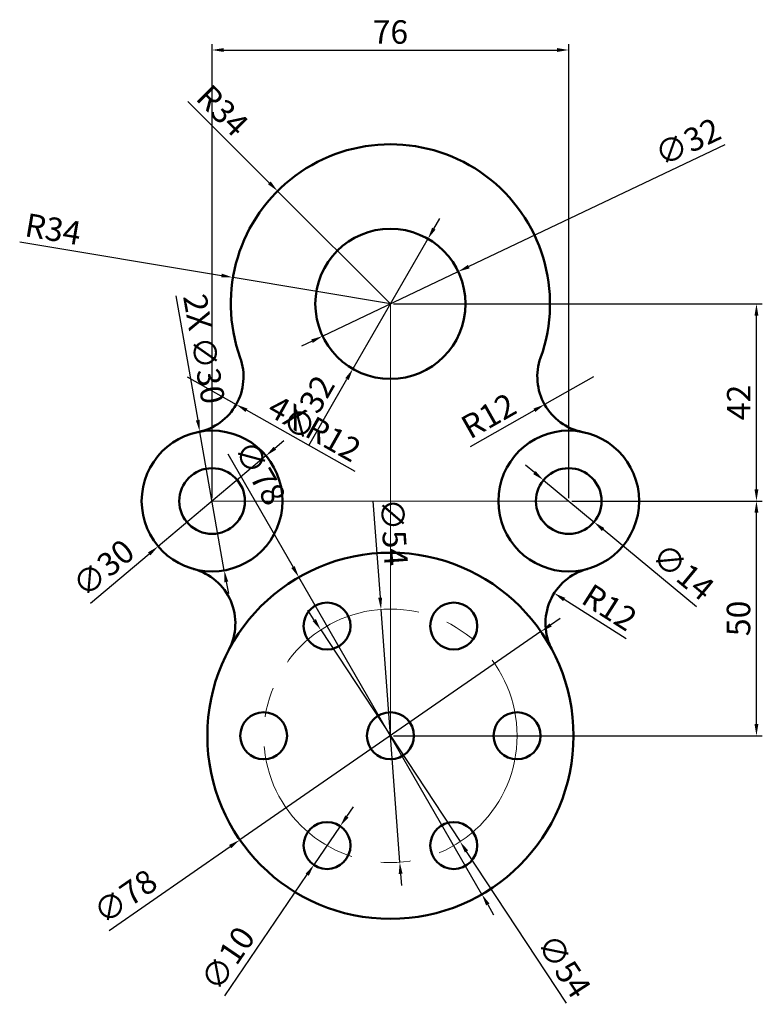
# Model space of a CAD drawing. Units: millimetres. Extents: x 2281 to 2439, y 1720 to 1930.
import ezdxf

# ---------------------------------------------------------------- set-up
doc = ezdxf.new("R2010")
doc.units = ezdxf.units.MM
doc.linetypes.add('CENTER', pattern=[50.8, 31.75, -6.35, 6.35, -6.35])
for name, color, linetype, lineweight in [('M-CNTR', 4, 'CENTER', 18), ('M-CONS', 8, 'Continuous', 13), ('M-DIMS', 2, 'Continuous', 25), ('M-OUTL', 7, 'Continuous', 50)]:
    doc.layers.add(name, color=color, linetype=linetype, lineweight=lineweight)
doc.styles.get("Standard").update_dxf_attribs({"font": 'arial.ttf'})
doc.dimstyles.new('ISO-25', dxfattribs={"dimtxt": 5, "dimasz": 2.5, "dimexe": 1.25, "dimexo": 0.625, "dimtad": 1, "dimtxsty": 'Standard', "dimcen": 2.5, "dimadec": 0, "dimazin": 0, "dimtfac": 1, "dimtmove": 0, "dimatfit": 3, "dimfxl": 1, "dimarcsym": 0})

# ---------------------------------------------------------------- blocks, each defined once
blk = doc.blocks.new('*U1')
blk.add_circle((0, 0), 5)
blk = doc.blocks.new('*U2')
at = {"layer": 'M-OUTL', "color": 0, "linetype": 'ByBlock', "lineweight": -2, "transparency": 16777216}
for p, rotation in [((2346.54, 1801.05), 119.9999999999999), ((2373.54, 1801.05), 59.99999999999997), ((2333.04, 1777.67), 180), ((2346.54, 1754.29), 239.9999999999999), ((2373.54, 1754.29), 299.9999999999999)]:
    blk.add_blockref('*U1', p, dxfattribs=dict(at, rotation=rotation))
blk.add_blockref('*U1', (2387.04, 1777.67), dxfattribs=at)
blk = doc.blocks.new('*D3')
at = {"layer": 'Defpoints', "color": 0, "transparency": 16777216}
for p in [(2398.04, 1923.75), (2322.04, 1827.67), (2398.04, 1827.67)]:
    blk.add_point(p, dxfattribs=at)
at = {"layer": 'M-DIMS', "color": 0, "lineweight": -2, "transparency": 16777216}
for p, q in [((2322.04, 1828.29), (2322.04, 1925)), ((2324.54, 1923.75), (2395.54, 1923.75)), ((2398.04, 1828.29), (2398.04, 1925))]:
    blk.add_line(p, q, dxfattribs=at)
at = {"layer": 'M-DIMS', "color": 0, "transparency": 16777216}
for points in [[(2324.54, 1924.16), (2324.54, 1923.33), (2322.04, 1923.75)], [(2395.54, 1924.16), (2395.54, 1923.33), (2398.04, 1923.75)]]:
    blk.add_solid(points, dxfattribs=at)
at = {"layer": 'M-DIMS', "color": 0, "transparency": 16777216, "insert": (2360.04, 1926.93), "char_height": 5, "attachment_point": 5}
blk.add_mtext('76', dxfattribs=at)
blk = doc.blocks.new('*D4')
at = {"layer": 'Defpoints', "color": 0, "transparency": 16777216}
for p in [(2398.04, 1827.67), (2438.04, 1827.67), (2360.04, 1777.67)]:
    blk.add_point(p, dxfattribs=at)
at = {"layer": 'M-DIMS', "color": 0, "lineweight": -2, "transparency": 16777216}
for p, q in [((2398.67, 1827.67), (2439.29, 1827.67)), ((2438.04, 1780.17), (2438.04, 1825.17)), ((2360.67, 1777.67), (2439.29, 1777.67))]:
    blk.add_line(p, q, dxfattribs=at)
at = {"layer": 'M-DIMS', "color": 0, "transparency": 16777216}
for points in [[(2437.62, 1825.17), (2438.45, 1825.17), (2438.04, 1827.67)], [(2437.62, 1780.17), (2438.45, 1780.17), (2438.04, 1777.67)]]:
    blk.add_solid(points, dxfattribs=at)
at = {"layer": 'M-DIMS', "color": 0, "transparency": 16777216, "insert": (2434.86, 1802.67), "char_height": 5, "attachment_point": 5, "rotation": 90}
blk.add_mtext('50', dxfattribs=at)
blk = doc.blocks.new('*D5')
at = {"layer": 'Defpoints', "color": 0, "transparency": 16777216}
for p in [(2360.04, 1869.67), (2438.04, 1869.67), (2398.04, 1827.67)]:
    blk.add_point(p, dxfattribs=at)
at = {"layer": 'M-DIMS', "color": 0, "lineweight": -2, "transparency": 16777216}
for p, q in [((2360.67, 1869.67), (2439.29, 1869.67)), ((2438.04, 1830.17), (2438.04, 1867.17)), ((2398.67, 1827.67), (2439.29, 1827.67))]:
    blk.add_line(p, q, dxfattribs=at)
at = {"layer": 'M-DIMS', "color": 0, "transparency": 16777216}
for points in [[(2437.62, 1867.17), (2438.45, 1867.17), (2438.04, 1869.67)], [(2437.62, 1830.17), (2438.45, 1830.17), (2438.04, 1827.67)]]:
    blk.add_solid(points, dxfattribs=at)
at = {"layer": 'M-DIMS', "color": 0, "transparency": 16777216, "insert": (2434.9, 1848.67), "char_height": 5, "attachment_point": 5, "rotation": 90}
blk.add_mtext('42', dxfattribs=at)
blk = doc.blocks.new('*D6')
at = {"layer": 'Defpoints', "color": 0, "transparency": 16777216}
for p in [(2333.53, 1837.32), (2310.56, 1818.02)]:
    blk.add_point(p, dxfattribs=at)
at = {"layer": 'M-DIMS', "color": 0, "lineweight": -2, "transparency": 16777216}
for p, q in [((2335.44, 1838.93), (2337.35, 1840.54)), ((2333.53, 1837.32), (2310.56, 1818.02)), ((2296.14, 1805.9), (2308.65, 1816.41))]:
    blk.add_line(p, q, dxfattribs=at)
at = {"layer": 'M-DIMS', "color": 0, "transparency": 16777216}
for points in [[(2335.17, 1839.25), (2335.71, 1838.61), (2333.53, 1837.32)], [(2308.38, 1816.73), (2308.91, 1816.09), (2310.56, 1818.02)]]:
    blk.add_solid(points, dxfattribs=at)
at = {"layer": 'M-DIMS', "color": 0, "transparency": 16777216, "insert": (2299.3, 1812.89), "char_height": 5, "attachment_point": 5, "rotation": 40.0457}
blk.add_mtext('∅30', dxfattribs=at)
blk = doc.blocks.new('*D7')
at = {"layer": 'Defpoints', "color": 0, "transparency": 16777216}
for p in [(2392.65, 1832.14), (2403.43, 1823.2)]:
    blk.add_point(p, dxfattribs=at)
at = {"layer": 'M-DIMS', "color": 0, "lineweight": -2, "transparency": 16777216}
for p, q in [((2390.73, 1833.73), (2388.8, 1835.33)), ((2392.65, 1832.14), (2403.43, 1823.2)), ((2425.23, 1805.14), (2405.36, 1821.61))]:
    blk.add_line(p, q, dxfattribs=at)
at = {"layer": 'M-DIMS', "color": 0, "transparency": 16777216}
for points in [[(2390.99, 1834.05), (2390.46, 1833.41), (2392.65, 1832.14)], [(2405.62, 1821.93), (2405.09, 1821.29), (2403.43, 1823.2)]]:
    blk.add_solid(points, dxfattribs=at)
at = {"layer": 'M-DIMS', "color": 0, "transparency": 16777216, "insert": (2422.02, 1812.11), "char_height": 5, "attachment_point": 5, "rotation": 320.3492}
blk.add_mtext('∅14', dxfattribs=at)
blk = doc.blocks.new('*D8')
at = {"layer": 'Defpoints', "color": 0, "transparency": 16777216}
for p in [(2345.2, 1800.22), (2374.89, 1755.12)]:
    blk.add_point(p, dxfattribs=at)
at = {"layer": 'M-DIMS', "color": 0, "lineweight": -2, "transparency": 16777216}
for p, q in [((2343.83, 1802.31), (2342.45, 1804.4)), ((2345.2, 1800.22), (2374.89, 1755.12)), ((2397.55, 1720.68), (2376.26, 1753.03))]:
    blk.add_line(p, q, dxfattribs=at)
at = {"layer": 'M-DIMS', "color": 0, "transparency": 16777216}
for points in [[(2344.17, 1802.54), (2343.48, 1802.08), (2345.2, 1800.22)], [(2376.61, 1753.26), (2375.91, 1752.8), (2374.89, 1755.12)]]:
    blk.add_solid(points, dxfattribs=at)
at = {"layer": 'M-DIMS', "color": 0, "transparency": 16777216, "insert": (2396.52, 1728.28), "char_height": 5, "attachment_point": 5, "rotation": 303.3505}
blk.add_mtext('∅54', dxfattribs=at)
blk = doc.blocks.new('*D9')
at = {"layer": 'Defpoints', "color": 0, "transparency": 16777216}
for p in [(2392.12, 1799.85), (2327.96, 1755.49)]:
    blk.add_point(p, dxfattribs=at)
at = {"layer": 'M-DIMS', "color": 0, "lineweight": -2, "transparency": 16777216}
for p, q in [((2394.18, 1801.27), (2396.24, 1802.69)), ((2392.12, 1799.85), (2327.96, 1755.49)), ((2300.09, 1736.22), (2325.91, 1754.07))]:
    blk.add_line(p, q, dxfattribs=at)
at = {"layer": 'M-DIMS', "color": 0, "transparency": 16777216}
for points in [[(2393.94, 1801.61), (2394.42, 1800.93), (2392.12, 1799.85)], [(2325.67, 1754.41), (2326.14, 1753.73), (2327.96, 1755.49)]]:
    blk.add_solid(points, dxfattribs=at)
at = {"layer": 'M-DIMS', "color": 0, "transparency": 16777216, "insert": (2303.9, 1742.89), "char_height": 5, "attachment_point": 5, "rotation": 34.6572}
blk.add_mtext('∅78', dxfattribs=at)
blk = doc.blocks.new('*D10')
at = {"layer": 'Defpoints', "color": 0, "transparency": 16777216}
for p in [(2349.36, 1758.42), (2343.73, 1750.15)]:
    blk.add_point(p, dxfattribs=at)
at = {"layer": 'M-DIMS', "color": 0, "lineweight": -2, "transparency": 16777216}
for p, q in [((2350.76, 1760.49), (2352.17, 1762.56)), ((2349.36, 1758.42), (2343.73, 1750.15)), ((2324.76, 1722.26), (2342.33, 1748.09))]:
    blk.add_line(p, q, dxfattribs=at)
at = {"layer": 'M-DIMS', "color": 0, "transparency": 16777216}
for points in [[(2350.42, 1760.72), (2351.11, 1760.25), (2349.36, 1758.42)], [(2341.98, 1748.32), (2342.67, 1747.85), (2343.73, 1750.15)]]:
    blk.add_solid(points, dxfattribs=at)
at = {"layer": 'M-DIMS', "color": 0, "transparency": 16777216, "insert": (2325.91, 1729.85), "char_height": 5, "attachment_point": 5, "rotation": 55.7774}
blk.add_mtext('∅10', dxfattribs=at)
blk = doc.blocks.new('*D11')
at = {"layer": 'Defpoints', "color": 0, "transparency": 16777216}
for p in [(2374.49, 1876.54), (2345.59, 1862.8)]:
    blk.add_point(p, dxfattribs=at)
at = {"layer": 'M-DIMS', "color": 0, "lineweight": -2, "transparency": 16777216}
for p, q in [((2431.32, 1903.57), (2376.75, 1877.62)), ((2345.59, 1862.8), (2374.49, 1876.54)), ((2343.34, 1861.72), (2341.08, 1860.65))]:
    blk.add_line(p, q, dxfattribs=at)
at = {"layer": 'M-DIMS', "color": 0, "transparency": 16777216}
for points in [[(2376.57, 1877.99), (2376.93, 1877.24), (2374.49, 1876.54)], [(2343.16, 1862.1), (2343.52, 1861.35), (2345.59, 1862.8)]]:
    blk.add_solid(points, dxfattribs=at)
at = {"layer": 'M-DIMS', "color": 0, "transparency": 16777216, "insert": (2423.66, 1903.6), "char_height": 5, "attachment_point": 5, "rotation": 25.4378}
blk.add_mtext('∅32', dxfattribs=at)
blk = doc.blocks.new('*D12')
at = {"layer": 'Defpoints', "color": 0, "transparency": 16777216}
for p in [(2326.51, 1875.29), (2360.04, 1869.67)]:
    blk.add_point(p, dxfattribs=at)
at = {"layer": 'M-DIMS', "color": 0, "lineweight": -2, "transparency": 16777216}
for p, q in [((2281.05, 1882.91), (2324.05, 1875.7)), ((2360.04, 1869.67), (2326.51, 1875.29))]:
    blk.add_line(p, q, dxfattribs=at)
at = {"layer": 'M-DIMS', "color": 0, "transparency": 16777216}
blk.add_solid([(2324.11, 1876.11), (2323.98, 1875.29), (2326.51, 1875.29)], dxfattribs=at)
at = {"layer": 'M-DIMS', "color": 0, "transparency": 16777216, "insert": (2288.08, 1884.96), "char_height": 5, "attachment_point": 5, "rotation": 350.4857}
blk.add_mtext('R34', dxfattribs=at)
blk = doc.blocks.new('*D13')
at = {"layer": 'Defpoints', "color": 0, "transparency": 16777216}
for p in [(2394.95, 1808.04), (2405.08, 1801.6)]:
    blk.add_point(p, dxfattribs=at)
at = {"layer": 'M-DIMS', "color": 0, "lineweight": -2, "transparency": 16777216}
blk.add_line((2410.27, 1798.31), (2397.06, 1806.7), dxfattribs=at)
at = {"layer": 'M-DIMS', "color": 0, "transparency": 16777216}
blk.add_solid([(2397.29, 1807.05), (2396.84, 1806.35), (2394.95, 1808.04)], dxfattribs=at)
at = {"layer": 'M-DIMS', "color": 0, "transparency": 16777216, "insert": (2406.4, 1804.48), "char_height": 5, "attachment_point": 5, "rotation": 327.5537}
blk.add_mtext('R12', dxfattribs=at)
blk = doc.blocks.new('*D14')
at = {"layer": 'Defpoints', "color": 0, "transparency": 16777216}
for p in [(2403.34, 1854.14), (2392.9, 1848.24)]:
    blk.add_point(p, dxfattribs=at)
at = {"layer": 'M-DIMS', "color": 0, "lineweight": -2, "transparency": 16777216}
for p, q in [((2403.34, 1854.14), (2392.9, 1848.24)), ((2377.1, 1839.31), (2390.72, 1847.01))]:
    blk.add_line(p, q, dxfattribs=at)
at = {"layer": 'M-DIMS', "color": 0, "transparency": 16777216}
blk.add_solid([(2390.52, 1847.37), (2390.93, 1846.65), (2392.9, 1848.24)], dxfattribs=at)
at = {"layer": 'M-DIMS', "color": 0, "transparency": 16777216, "insert": (2381.28, 1845.27), "char_height": 5, "attachment_point": 5, "rotation": 29.4763}
blk.add_mtext('R12', dxfattribs=at)
blk = doc.blocks.new('MOUNTING-BOSS-30-BORE-14')
for radius in [15, 7]:
    blk.add_circle((0, 0), radius)
blk = doc.blocks.new('*D16')
at = {"layer": 'Defpoints', "color": 0, "transparency": 16777216}
for p in [(2336, 1893.71), (2360.04, 1869.67)]:
    blk.add_point(p, dxfattribs=at)
at = {"layer": 'M-DIMS', "color": 0, "lineweight": -2, "transparency": 16777216}
for p, q in [((2316.91, 1912.79), (2334.23, 1895.48)), ((2360.04, 1869.67), (2336, 1893.71))]:
    blk.add_line(p, q, dxfattribs=at)
at = {"layer": 'M-DIMS', "color": 0, "transparency": 16777216}
blk.add_solid([(2334.53, 1895.77), (2333.94, 1895.18), (2336, 1893.71)], dxfattribs=at)
at = {"layer": 'M-DIMS', "color": 0, "transparency": 16777216, "insert": (2323.82, 1910.38), "char_height": 5, "attachment_point": 5, "rotation": 315.0052}
blk.add_mtext('R34', dxfattribs=at)
blk = doc.blocks.new('*D17')
at = {"layer": 'Defpoints', "color": 0, "transparency": 16777216}
for p in [(2368.04, 1883.53), (2352.04, 1855.81)]:
    blk.add_point(p, dxfattribs=at)
at = {"layer": 'M-DIMS', "color": 0, "lineweight": -2, "transparency": 16777216}
for p, q in [((2369.29, 1885.69), (2370.54, 1887.86)), ((2368.04, 1883.53), (2352.04, 1855.81)), ((2342.64, 1839.53), (2350.79, 1853.65))]:
    blk.add_line(p, q, dxfattribs=at)
at = {"layer": 'M-DIMS', "color": 0, "transparency": 16777216}
for points in [[(2368.93, 1885.9), (2369.65, 1885.48), (2368.04, 1883.53)], [(2350.43, 1853.86), (2351.15, 1853.44), (2352.04, 1855.81)]]:
    blk.add_solid(points, dxfattribs=at)
at = {"layer": 'M-DIMS', "color": 0, "transparency": 16777216, "insert": (2343.22, 1847.17), "char_height": 5, "attachment_point": 5, "rotation": 60.0001}
blk.add_mtext('∅32', dxfattribs=at)
blk = doc.blocks.new('*D18')
at = {"layer": 'Defpoints', "color": 0, "transparency": 16777216}
for p in [(2316.74, 1854.14), (2327.19, 1848.24)]:
    blk.add_point(p, dxfattribs=at)
at = {"layer": 'M-DIMS', "color": 0, "lineweight": -2, "transparency": 16777216}
for p, q in [((2316.74, 1854.14), (2327.19, 1848.24)), ((2352.52, 1833.93), (2329.37, 1847.01))]:
    blk.add_line(p, q, dxfattribs=at)
at = {"layer": 'M-DIMS', "color": 0, "transparency": 16777216}
blk.add_solid([(2329.57, 1847.37), (2329.16, 1846.65), (2327.19, 1848.24)], dxfattribs=at)
at = {"layer": 'M-DIMS', "color": 0, "transparency": 16777216, "insert": (2343.57, 1842.58), "char_height": 5, "attachment_point": 5, "rotation": 330.5267}
blk.add_mtext('4X R12', dxfattribs=at)
blk = doc.blocks.new('*D19')
at = {"layer": 'Defpoints', "color": 0, "transparency": 16777216}
for p in [(2319.44, 1842.44), (2324.65, 1812.9)]:
    blk.add_point(p, dxfattribs=at)
at = {"layer": 'M-DIMS', "color": 0, "lineweight": -2, "transparency": 16777216}
for p, q in [((2314.34, 1871.39), (2319.01, 1844.9)), ((2324.65, 1812.9), (2319.44, 1842.44)), ((2325.08, 1810.44), (2325.52, 1807.97))]:
    blk.add_line(p, q, dxfattribs=at)
at = {"layer": 'M-DIMS', "color": 0, "transparency": 16777216}
for points in [[(2319.42, 1844.98), (2318.6, 1844.83), (2319.44, 1842.44)], [(2325.49, 1810.51), (2324.67, 1810.36), (2324.65, 1812.9)]]:
    blk.add_solid(points, dxfattribs=at)
at = {"layer": 'M-DIMS', "color": 0, "transparency": 16777216, "insert": (2319.72, 1859.96), "char_height": 5, "attachment_point": 5, "rotation": 279.997}
blk.add_mtext('2X ∅30', dxfattribs=at)
blk = doc.blocks.new('*D20')
at = {"layer": 'Defpoints', "color": 0, "transparency": 16777216}
for p in [(2340.54, 1811.44), (2379.54, 1743.89)]:
    blk.add_point(p, dxfattribs=at)
at = {"layer": 'M-DIMS', "color": 0, "lineweight": -2, "transparency": 16777216}
for p, q in [((2325.38, 1837.71), (2339.29, 1813.61)), ((2379.54, 1743.89), (2340.54, 1811.44)), ((2380.79, 1741.73), (2382.04, 1739.56))]:
    blk.add_line(p, q, dxfattribs=at)
at = {"layer": 'M-DIMS', "color": 0, "transparency": 16777216}
for points in [[(2339.65, 1813.82), (2338.93, 1813.4), (2340.54, 1811.44)], [(2381.15, 1741.94), (2380.43, 1741.52), (2379.54, 1743.89)]]:
    blk.add_solid(points, dxfattribs=at)
at = {"layer": 'M-DIMS', "color": 0, "transparency": 16777216, "insert": (2331.72, 1833.37), "char_height": 5, "attachment_point": 5, "rotation": 299.9993}
blk.add_mtext('∅78', dxfattribs=at)
blk = doc.blocks.new('*D21')
at = {"layer": 'Defpoints', "color": 0, "transparency": 16777216}
for p in [(2358.04, 1804.6), (2362.04, 1750.74)]:
    blk.add_point(p, dxfattribs=at)
at = {"layer": 'M-DIMS', "color": 0, "lineweight": -2, "transparency": 16777216}
for p, q in [((2356.33, 1827.65), (2357.86, 1807.09)), ((2362.04, 1750.74), (2358.04, 1804.6)), ((2362.23, 1748.25), (2362.41, 1745.76))]:
    blk.add_line(p, q, dxfattribs=at)
at = {"layer": 'M-DIMS', "color": 0, "transparency": 16777216}
for points in [[(2358.27, 1807.12), (2357.44, 1807.06), (2358.04, 1804.6)], [(2362.64, 1748.28), (2361.81, 1748.22), (2362.04, 1750.74)]]:
    blk.add_solid(points, dxfattribs=at)
at = {"layer": 'M-DIMS', "color": 0, "transparency": 16777216, "insert": (2360.15, 1821), "char_height": 5, "attachment_point": 5, "rotation": 274.2471}
blk.add_mtext('∅54', dxfattribs=at)

msp = doc.modelspace()

# ---------------------------------------------------------------- linework, layer by layer
at = {"layer": 'M-CNTR'}
msp.add_circle((2360.044, 1777.67), 27, dxfattribs=at)
at = {"layer": 'M-CONS'}
for p, q in [((2360.044, 1827.67), (2360.044, 1869.67)), ((2360.044, 1827.67), (2322.044, 1827.67)), ((2360.044, 1777.67), (2360.044, 1827.67)), ((2360.044, 1827.67), (2398.044, 1827.67))]:
    msp.add_line(p, q, dxfattribs=at)
at = {"layer": 'M-OUTL'}
for centre, radius in [((2360.044, 1869.67), 16), ((2360.044, 1777.67), 39), ((2360.044, 1777.67), 5)]:
    msp.add_circle(centre, radius, dxfattribs=at)
for centre, radius, start, end in [((2360.044, 1869.67), 34, 340.27476, 199.72524), ((2316.743, 1854.144), 12, 281.32221, 19.72524), ((2403.344, 1854.144), 12, 160.27476, 258.67779), ((2315.008, 1801.603), 12, 332.01302, 74.89529), ((2405.079, 1801.603), 12, 105.10471, 207.98698)]:
    msp.add_arc(centre, radius, start, end, dxfattribs=at)

# ---------------------------------------------------------------- block references
for name, p in [('MOUNTING-BOSS-30-BORE-14', (2322.044, 1827.67)), ('MOUNTING-BOSS-30-BORE-14', (2398.044, 1827.67)), ('*U2', (0, 0))]:
    msp.add_blockref(name, p, dxfattribs=at)

# ---------------------------------------------------------------- dimensions: what is measured, and where the dimension line sits
at = {"layer": 'M-DIMS'}
dim = msp.add_linear_dim(base=(2398.044, 1923.747), p1=(2322.044, 1827.67), p2=(2398.044, 1827.67), dimstyle='ISO-25', override={"dimclrd": 0, "dimclre": 0, "dimclrt": 0}, dxfattribs=at)
dim.commit()
dim.dimension.update_dxf_attribs({"geometry": '*D3', "text_midpoint": (2360.044, 1926.925)})
for center, mpoint, override, picture, middle in [((2360.044, 1869.67), (2336, 1893.709), {"dimdec": 0, "dimlfac": 1, "dimrnd": 0, "dimzin": 0, "dimdsep": 46, "dimlunit": 2}, '*D16', (2321.573, 1908.133)), ((2360.044, 1869.67), (2326.511, 1875.29), {"dimclrd": 0, "dimclre": 0, "dimclrt": 0}, '*D12', (2287.552, 1881.819)), ((2405.079, 1801.603), (2394.953, 1808.041), {"dimclrd": 0, "dimclre": 0, "dimclrt": 0}, '*D13', (2404.719, 1801.832))]:
    dim = msp.add_radius_dim(center=center, mpoint=mpoint, dimstyle='ISO-25', override=override, dxfattribs=at)
    dim.commit()
    dim.dimension.update_dxf_attribs({"geometry": picture, "text_midpoint": middle, "dimtype": 164})
for p1, p2, override, picture, middle in [((2345.595, 1862.797), (2374.492, 1876.542), {"dimclrd": 0, "dimclre": 0, "dimclrt": 0}, '*D11', (2425.084, 1900.606)), ((2379.543, 1743.895), (2340.544, 1811.445), {"dimdec": 0, "dimlfac": 1, "dimrnd": 0, "dimzin": 0, "dimdsep": 46, "dimlunit": 2}, '*D20', (2328.844, 1831.71)), ((2392.654, 1832.137), (2403.433, 1823.203), {"dimclrd": 0, "dimclre": 0, "dimclrt": 0}, '*D7', (2419.905, 1809.552)), ((2362.043, 1750.744), (2358.044, 1804.596), {"dimdec": 0, "dimlfac": 1, "dimrnd": 0, "dimzin": 0, "dimdsep": 46, "dimlunit": 2}, '*D21', (2356.844, 1820.751)), ((2345.2, 1800.224), (2374.887, 1755.116), {"dimclrd": 0, "dimclre": 0, "dimclrt": 0}, '*D8', (2393.747, 1726.459)), ((2392.124, 1799.848), (2327.963, 1755.492), {"dimclrd": 0, "dimclre": 0, "dimclrt": 0}, '*D9', (2305.791, 1740.164)), ((2349.356, 1758.421), (2343.732, 1750.153), {"dimclrd": 0, "dimclre": 0, "dimclrt": 0}, '*D10', (2328.651, 1727.982))]:
    dim = msp.add_diameter_dim_2p(p1=p1, p2=p2, dimstyle='ISO-25', override=override, dxfattribs=at)
    dim.commit()
    dim.dimension.update_dxf_attribs({"geometry": picture, "text_midpoint": middle, "dimtype": 163})
for p1, p2, override, picture, middle in [((2368.044, 1883.526), (2352.044, 1855.813), {"dimdec": 0, "dimlfac": 1, "dimrnd": 0, "dimzin": 0, "dimdsep": 46, "dimlunit": 2}, '*D17', (2346.093, 1845.507)), ((2333.527, 1837.321), (2310.561, 1818.019), {"dimclrd": 0, "dimclre": 0, "dimclrt": 0}, '*D6', (2299.303, 1812.891))]:
    dim = msp.add_diameter_dim_2p(p1=p1, p2=p2, dimstyle='ISO-25', override=override, dxfattribs=at)
    dim.commit()
    dim.dimension.update_dxf_attribs({"geometry": picture, "text_midpoint": middle})
dim = msp.add_diameter_dim_2p(p1=(2324.648, 1812.898), p2=(2319.44, 1842.442), text='2X <>', dimstyle='ISO-25', override={"dimdec": 0, "dimlfac": 1, "dimrnd": 0, "dimzin": 0, "dimdsep": 46, "dimlunit": 2}, dxfattribs=at)
dim.commit()
dim.dimension.update_dxf_attribs({"geometry": '*D19', "text_midpoint": (2316.454, 1859.38), "dimtype": 163})
for base, p1, p2, picture, middle in [((2438.036, 1869.67), (2398.044, 1827.67), (2360.044, 1869.67), '*D5', (2434.901, 1848.67)), ((2438.036, 1827.67), (2360.044, 1777.67), (2398.044, 1827.67), '*D4', (2434.858, 1802.67))]:
    dim = msp.add_linear_dim(base=base, p1=p1, p2=p2, angle=90, dimstyle='ISO-25', override={"dimclrd": 0, "dimclre": 0, "dimclrt": 0}, dxfattribs=at)
    dim.commit()
    dim.dimension.update_dxf_attribs({"geometry": picture, "text_midpoint": middle})
dim = msp.add_radius_dim(center=(2316.743, 1854.144), mpoint=(2327.19, 1848.24), text='4X <>', dimstyle='ISO-25', override={"dimdec": 0, "dimlfac": 1, "dimrnd": 0, "dimzin": 0, "dimdsep": 46, "dimlunit": 2}, dxfattribs=at)
dim.commit()
dim.dimension.update_dxf_attribs({"geometry": '*D18', "text_midpoint": (2343.573, 1842.584)})
dim = msp.add_radius_dim(center=(2403.344, 1854.144), mpoint=(2392.898, 1848.24), dimstyle='ISO-25', override={"dimclrd": 0, "dimclre": 0, "dimclrt": 0}, dxfattribs=at)
dim.commit()
dim.dimension.update_dxf_attribs({"geometry": '*D14', "text_midpoint": (2381.28, 1845.274)})

doc.saveas('drawing.dxf')
